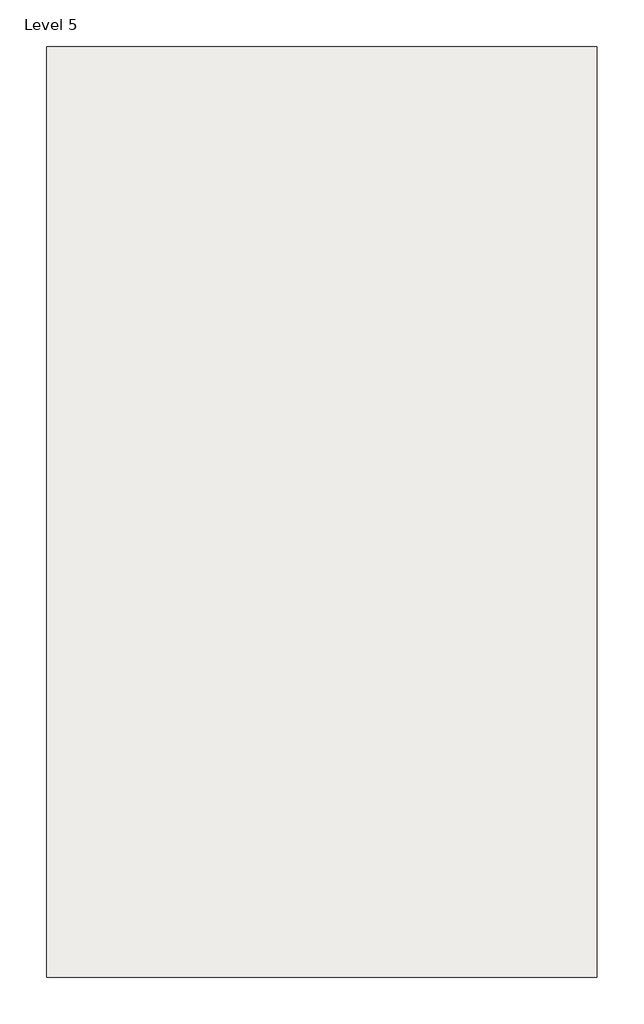
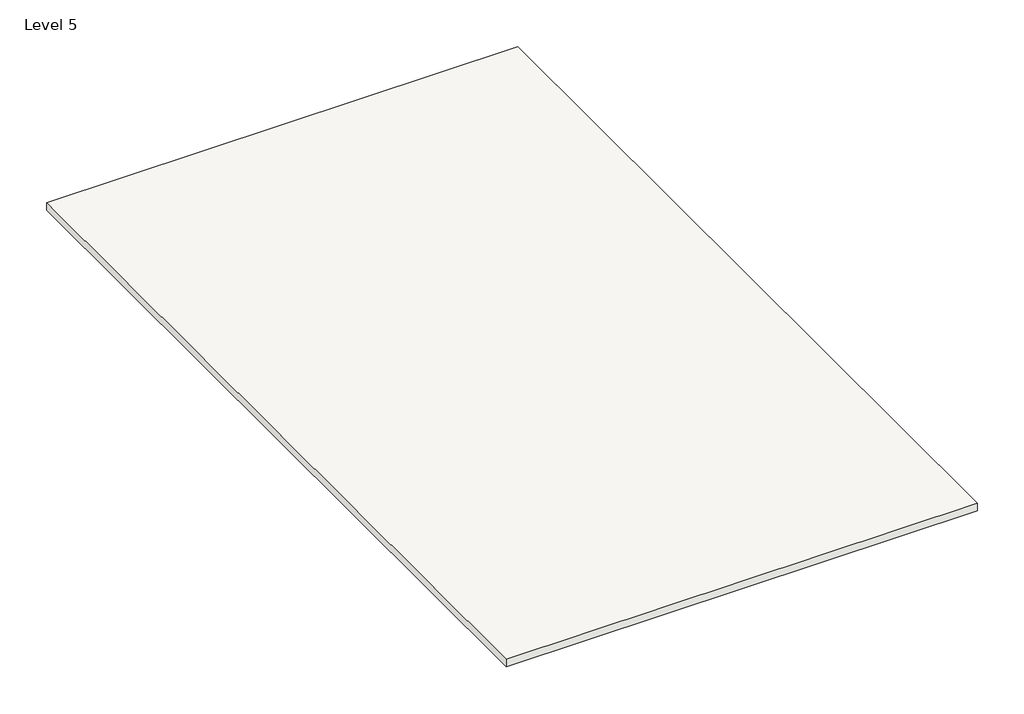
# One storey, incomplete: 1 slab.
"""IFC4 building model written with IfcOpenShell, lengths in millimetres."""

from ifc_helpers import new_model, si_unit, frame, origin, place, context, project, spatial, polyline, outline, extrude, element, save

model = new_model("IFC4")

# Units and contexts
model_context = context("Model", 3, world=origin())
ifc_project = project(units=[si_unit("LENGTHUNIT", "METRE", prefix="MILLI")], contexts=[model_context])

# Site, building, storey
site = spatial("IfcSite", under=ifc_project)
building = spatial("IfcBuilding", under=site)
storey = spatial("IfcBuildingStorey", under=building, Name="Level 5", Elevation=12192.0)

# Slab
placement = place(None, origin())
element("IfcSlab", 1, ObjectType="Generic - 12\"", at=placement, inside=storey, context=model_context, shape_type="SweptSolid", body=[
    extrude(outline(polyline([(9499.6, 15087.6), (9499.6, 152.4), (660.4, 152.4), (660.4, 15087.6), (9499.6, 15087.6)])), frame((0.0, 0.0, 12039.6), z_axis=(0.0, 0.0, 1.0), x_axis=(1.0, 0.0, 0.0)), (0.0, 0.0, 1.0), 152.4),
])

save(model, "model.ifc")

# Revit data of these elements
# Type "Generic - 12\""
#   Assembly Code = "B1010"
#   Function = 0
#   Layers, outside or top first: 0' - 6" no material (function 1)
# Element 1 (IfcSlab, "Generic - 12\"")
#   Height Offset From Level = 0' - 0"
#   Phase Created = New Construction
#   Materials on its faces: "Clad - White", "Default Floor"
# Materials
#   "Clad - White": class "Wood", colour RGB 242 242 238, transparency 0, Cost = 0
#   "Default Floor": colour RGB 128 128 128, transparency 0, Cost = 0
